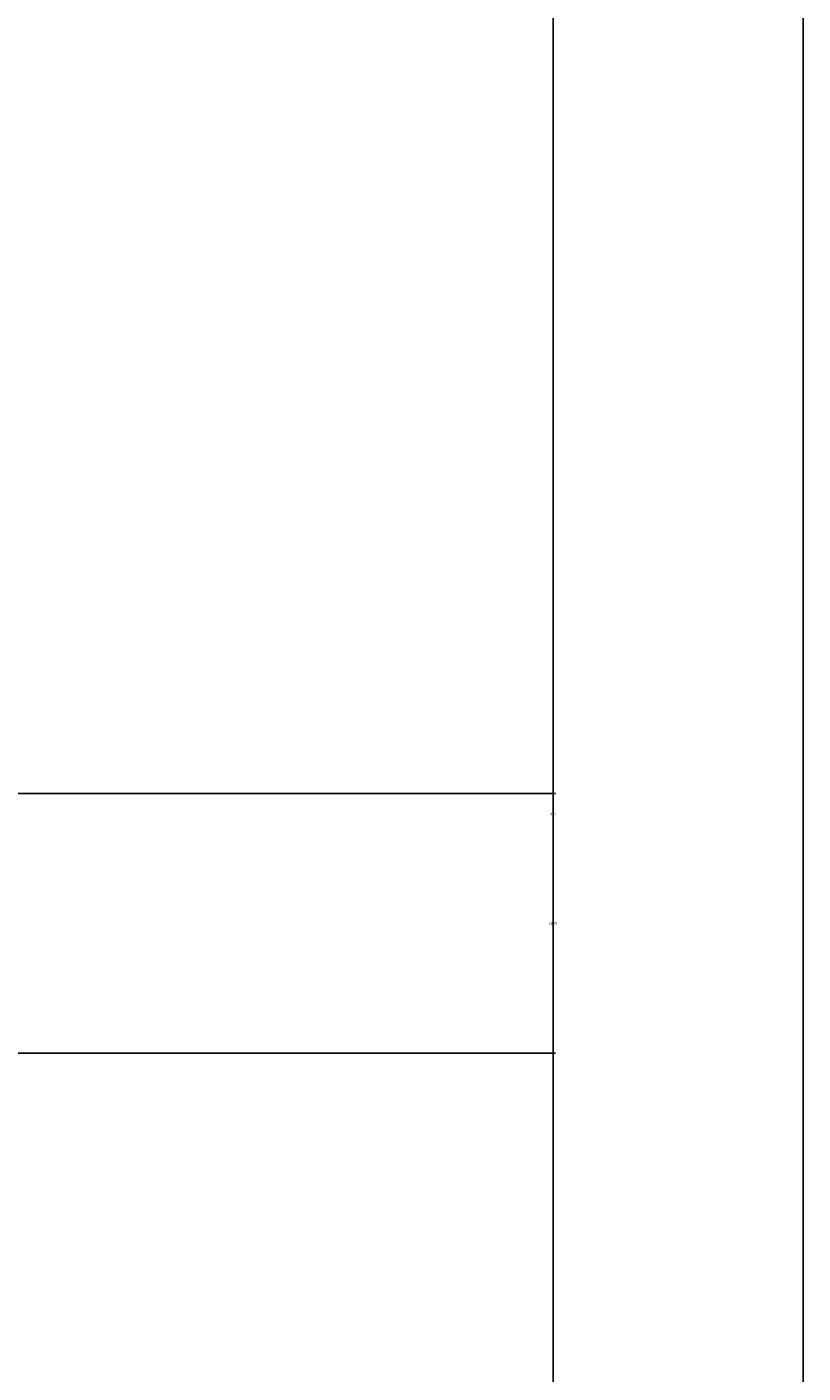
# Model space of a CAD drawing. Units: inches. Extents: x 1601 to 2297, y 1496 to 2631.
# Tile 32 of 57: x 2241 to 2297, y 2043 to 2141. Entities that reach past the tile are written whole.
import ezdxf

# ---------------------------------------------------------------- set-up
doc = ezdxf.new("R2010")
doc.units = ezdxf.units.IN
doc.layers.add('A-ANNO-DIMS', color=2, linetype='Continuous', lineweight=18)
doc.layers.add('A-ANNO-TTLB', color=7, linetype='Continuous', lineweight=25)
doc.styles.get("Standard").update_dxf_attribs({"font": 'arial.ttf'})
doc.dimstyles.get("Standard").update_dxf_attribs({"dimtxt": 0.18, "dimasz": 0.18, "dimexe": 0.18, "dimexo": 0.0625, "dimgap": 0.09, "dimtad": 0, "dimtih": 1, "dimtoh": 1, "dimdec": 4, "dimzin": 0, "dimdsep": 46, "dimtxsty": 'Standard', "dimcen": 0.09, "dimadec": 0, "dimazin": 0, "dimtfac": 1, "dimtdec": 4, "dimtofl": 0, "dimtmove": 0, "dimatfit": 3, "dimfxl": 1, "dimtolj": 1, "dimtzin": 0, "dimarcsym": 0})

# ---------------------------------------------------------------- blocks, each defined once
blk = doc.blocks.new('*D29')
at = {"layer": 'A-ANNO-DIMS', "color": 0, "lineweight": -2, "transparency": 16777216}
for p, q in [((2230.6, 2532.325), (2279.267, 2532.325)), ((2279.087, 2532.145), (2279.087, 2084.007)), ((2279.087, 1635.505), (2279.087, 2083.643)), ((2230.6, 1635.325), (2279.267, 1635.325))]:
    blk.add_line(p, q, dxfattribs=at)
at = {"layer": 'A-ANNO-DIMS', "color": 0, "transparency": 16777216}
for points in [[(2279.057, 2532.145), (2279.117, 2532.145), (2279.087, 2532.325)], [(2279.057, 1635.505), (2279.117, 1635.505), (2279.087, 1635.325)]]:
    blk.add_solid(points, dxfattribs=at)
at = {"layer": 'Defpoints', "color": 0, "transparency": 16777216}
for p in [(2230.537, 2532.325), (2279.087, 2532.325), (2230.537, 1635.325)]:
    blk.add_point(p, dxfattribs=at)
at = {"layer": 'A-ANNO-DIMS', "color": 0, "transparency": 16777216, "insert": (2279.087, 2083.825), "char_height": 0.18, "attachment_point": 5}
blk.add_mtext('\\A1;897', dxfattribs=at)
blk = doc.blocks.new('*D37')
at = {"layer": 'A-ANNO-DIMS', "color": 0, "lineweight": -2, "transparency": 16777216}
for p, q in [((2040.1, 2085.325), (2279.267, 2085.325)), ((2279.087, 2085.145), (2279.087, 2076.132)), ((2279.087, 2066.755), (2279.087, 2075.768)), ((2040.1, 2066.575), (2279.267, 2066.575))]:
    blk.add_line(p, q, dxfattribs=at)
at = {"layer": 'A-ANNO-DIMS', "color": 0, "transparency": 16777216}
for points in [[(2279.057, 2085.145), (2279.117, 2085.145), (2279.087, 2085.325)], [(2279.057, 2066.755), (2279.117, 2066.755), (2279.087, 2066.575)]]:
    blk.add_solid(points, dxfattribs=at)
at = {"layer": 'Defpoints', "color": 0, "transparency": 16777216}
for p in [(2040.037, 2085.325), (2279.087, 2085.325), (2040.037, 2066.575)]:
    blk.add_point(p, dxfattribs=at)
at = {"layer": 'A-ANNO-DIMS', "color": 0, "transparency": 16777216, "insert": (2279.087, 2075.95), "char_height": 0.18, "attachment_point": 5}
blk.add_mtext('\\A1;18.75', dxfattribs=at)

msp = doc.modelspace()

# ---------------------------------------------------------------- linework, layer by layer
at = {"layer": 'A-ANNO-TTLB'}
msp.add_lwpolyline([(1600.5933, 2631.1477), (2297.129, 2631.1477), (2297.129, 1496.1026), (1600.5933, 1496.1026)], close=True, dxfattribs=at)

# ---------------------------------------------------------------- dimensions: what is measured, and where the dimension line sits
at = {"layer": 'A-ANNO-DIMS'}
for base, p1, p2, override, picture, middle in [((2279.0873, 2532.3254), (2230.5373, 1635.3254), (2230.5373, 2532.3254), {"dimdec": 0, "dimlfac": 1, "dimrnd": 0, "dimzin": 0, "dimdsep": 46, "dimlunit": 2}, '*D29', (2279.0873, 2083.8254)), ((2279.0873, 2085.3254), (2040.0373, 2066.5754), (2040.0373, 2085.3254), {"dimdec": 2, "dimlfac": 1, "dimrnd": 0, "dimzin": 0, "dimdsep": 46, "dimlunit": 2}, '*D37', (2279.0873, 2075.9504))]:
    dim = msp.add_linear_dim(base=base, p1=p1, p2=p2, angle=90, dimstyle='Standard', override=override, dxfattribs=at)
    dim.commit()
    dim.dimension.update_dxf_attribs({"geometry": picture, "text_midpoint": middle})

doc.saveas('drawing.dxf')
